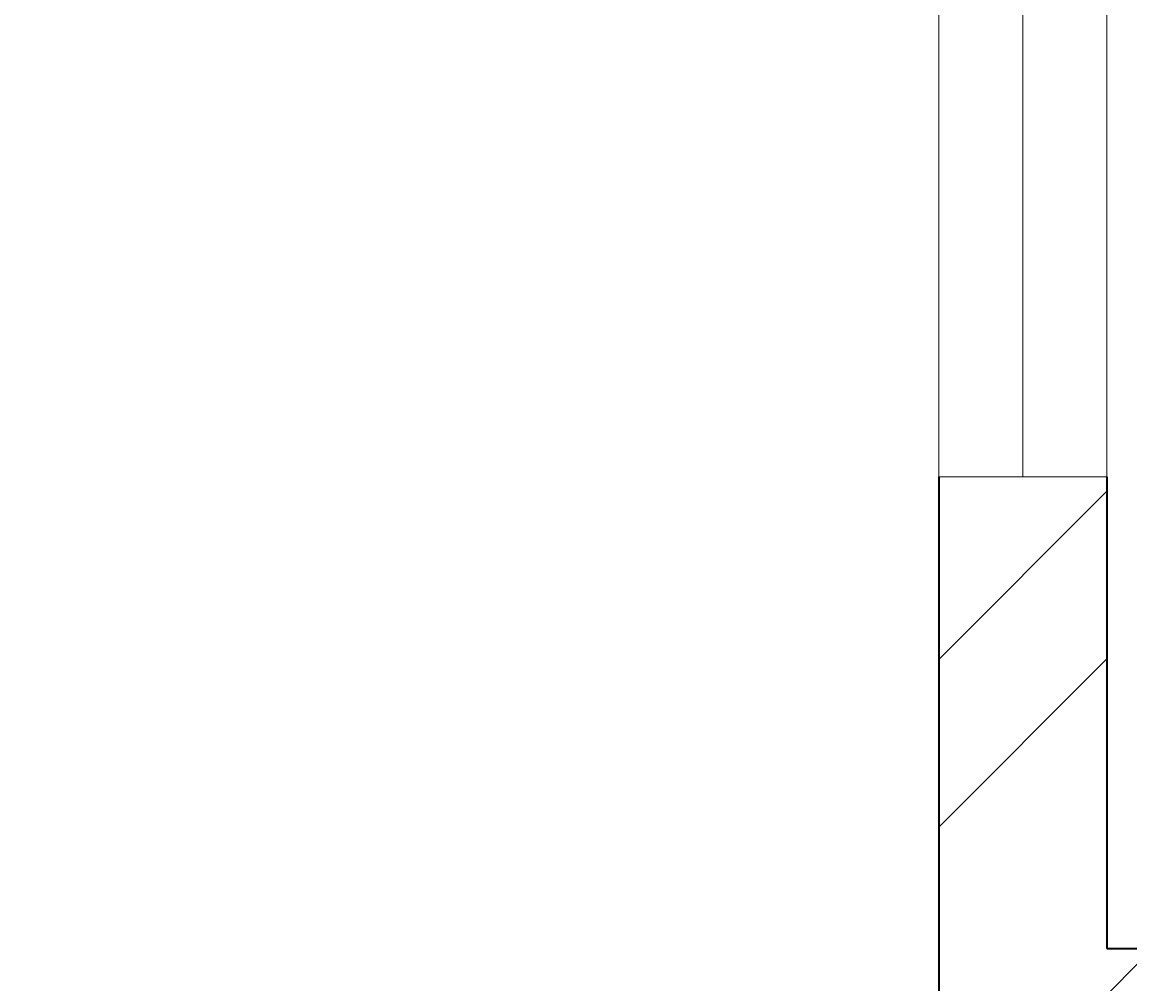
# Model space of a CAD drawing. Units: inches. Extents: x 1885 to 2748, y 783 to 2421.
# Tile 68 of 117: x 1992 to 2022, y 2022 to 2047. Entities that reach past the tile are written whole.
import ezdxf

# ---------------------------------------------------------------- set-up
doc = ezdxf.new("R2010")
doc.units = ezdxf.units.IN
for name, color, linetype, lineweight in [('A-ANNO-DIMS', 2, 'Continuous', 18), ('A-GLAZ', 181, 'Continuous', 18), ('A-WALL', 7, 'Continuous', 35)]:
    doc.layers.add(name, color=color, linetype=linetype, lineweight=lineweight)
doc.layers.add('A-WALL-PATT', color=85, linetype='Continuous', lineweight=13, true_color=0x58ba48)
doc.styles.get("Standard").update_dxf_attribs({"font": 'arial.ttf'})
doc.dimstyles.get("Standard").update_dxf_attribs({"dimtxt": 0.18, "dimasz": 0.18, "dimexe": 0.18, "dimexo": 0.0625, "dimgap": 0.09, "dimtad": 0, "dimtih": 1, "dimtoh": 1, "dimdec": 4, "dimzin": 0, "dimdsep": 46, "dimtxsty": 'Standard', "dimcen": 0.09, "dimadec": 0, "dimazin": 0, "dimtfac": 1, "dimtdec": 4, "dimtofl": 0, "dimtmove": 0, "dimatfit": 3, "dimfxl": 1, "dimtolj": 1, "dimtzin": 0, "dimarcsym": 0})

# ---------------------------------------------------------------- blocks, each defined once
blk = doc.blocks.new('*D48')
at = {"layer": 'A-ANNO-DIMS', "color": 0, "lineweight": -2, "transparency": 16777216}
for p, q in [((1980.711, 2348.006), (1902.844, 2348.006)), ((1903.024, 2347.826), (1903.024, 2114.937)), ((1903.024, 1881.686), (1903.024, 2114.574)), ((2016.711, 1881.506), (1902.844, 1881.506))]:
    blk.add_line(p, q, dxfattribs=at)
at = {"layer": 'A-ANNO-DIMS', "color": 0, "transparency": 16777216}
for points in [[(1902.994, 2347.826), (1903.054, 2347.826), (1903.024, 2348.006)], [(1902.994, 1881.686), (1903.054, 1881.686), (1903.024, 1881.506)]]:
    blk.add_solid(points, dxfattribs=at)
at = {"layer": 'Defpoints', "color": 0, "transparency": 16777216}
for p in [(1903.024, 2348.006), (1980.774, 2348.006), (2016.774, 1881.506)]:
    blk.add_point(p, dxfattribs=at)
at = {"layer": 'A-ANNO-DIMS', "color": 0, "transparency": 16777216, "insert": (1903.024, 2114.756), "char_height": 0.18, "attachment_point": 5}
blk.add_mtext('\\A1;466.5', dxfattribs=at)

msp = doc.modelspace()

# ---------------------------------------------------------------- hatches: boundary and pattern name
at = {"layer": 'A-WALL-PATT'}
h = msp.add_hatch(dxfattribs=at)
h.set_pattern_fill('ANSI32', color=256)
h.paths.add_polyline_path([(2007.772, 2318.006), (1980.774, 2318.006), (1980.774, 2281.215), (1985.274, 2281.215), (1985.274, 2313.506), (2007.772, 2313.506), (2007.772, 2315.756)])
h.paths.add_polyline_path([(2094.324, 2318.006), (2067.772, 2318.006), (2067.772, 2313.506), (2094.324, 2313.506), (2094.324, 2315.756)])
h.paths.add_polyline_path([(2131.367, 2315.756), (2131.367, 2318.006), (2131.189, 2318.006), (2112.609, 2318.006), (2112.609, 2313.506), (2117.274, 2313.506), (2117.274, 2255.201), (2121.774, 2255.201), (2121.774, 2313.506), (2131.367, 2313.506)])
h.paths.add_polyline_path([(2190.512, 2318.006), (2155.367, 2318.006), (2155.367, 2313.506), (2169.774, 2313.506), (2169.774, 2229.506), (2121.774, 2229.506), (2121.774, 2233.451), (2119.524, 2233.451), (2117.274, 2233.451), (2117.274, 2201.101), (2121.774, 2201.101), (2121.774, 2225.006), (2169.774, 2225.006), (2169.774, 2165.006), (2306.274, 2165.006), (2306.274, 2066.006), (2310.774, 2066.006), (2344.274, 2066.006), (2486.274, 2066.006), (2486.274, 1886.006), (2483.02, 1886.006), (2483.02, 1881.506), (2486.274, 1881.506), (2486.274, 1880.678), (2490.774, 1880.678), (2490.774, 2070.506), (2344.274, 2070.506), (2310.774, 2070.506), (2310.774, 2165.006), (2310.774, 2173.636), (2308.524, 2173.636), (2306.274, 2173.636), (2306.274, 2169.506), (2174.274, 2169.506), (2174.274, 2313.506), (2190.512, 2313.506), (2190.512, 2315.756)])
h.paths.add_polyline_path([(1985.274, 2221.215), (1980.774, 2221.215), (1980.774, 2165.006), (1992.774, 2165.006), (1992.774, 2141.927), (1997.274, 2141.927), (1997.274, 2165.006), (2117.274, 2165.006), (2117.274, 2163.126), (2121.774, 2163.126), (2121.774, 2172.734), (2119.524, 2172.734), (2117.274, 2172.734), (2117.274, 2169.506), (1985.274, 2169.506)])
h.paths.add_polyline_path([(1997.274, 2105.927), (1992.774, 2105.927), (1992.774, 2070.506), (2016.774, 2070.506), (2016.774, 2059.123), (2019.024, 2059.123), (2021.274, 2059.123), (2021.274, 2070.506), (2117.274, 2070.506), (2117.274, 2022.506), (2114.423, 2022.506), (2114.423, 2018.006), (2123.627, 2018.006), (2123.627, 2020.256), (2123.627, 2022.506), (2121.774, 2022.506), (2121.774, 2142.587), (2119.524, 2142.587), (2117.274, 2142.587), (2117.274, 2075.006), (1997.274, 2075.006)])
h.paths.add_polyline_path([(2092.029, 2020.256), (2092.029, 2022.506), (2021.274, 2022.506), (2021.274, 2035.123), (2016.774, 2035.123), (2016.774, 2018.006), (2016.774, 1978.784), (2021.274, 1978.784), (2021.274, 2018.006), (2092.029, 2018.006)])
h.paths.add_polyline_path([(2260.938, 2022.506), (2153.105, 2022.506), (2153.105, 2020.256), (2153.105, 2018.006), (2155.274, 2018.006), (2155.274, 1886.006), (2107.629, 1886.006), (2107.629, 1881.506), (2182.911, 1881.506), (2182.911, 1883.756), (2182.911, 1886.006), (2159.774, 1886.006), (2159.774, 2018.006), (2260.938, 2018.006), (2260.938, 2020.256)])
h.paths.add_polyline_path([(2047.629, 1883.756), (2047.629, 1886.006), (2021.274, 1886.006), (2021.274, 1918.784), (2019.024, 1918.784), (2016.774, 1918.784), (2016.774, 1881.506), (2047.629, 1881.506)])
h.paths.add_polyline_path([(2306.361, 1883.756), (2306.361, 1886.006), (2296.274, 1886.006), (2296.274, 1982.006), (2316.535, 1982.006), (2316.535, 1984.256), (2316.535, 1986.506), (2296.274, 1986.506), (2296.274, 2022.506), (2289.276, 2022.506), (2289.276, 2018.006), (2291.774, 2018.006), (2291.774, 1886.006), (2242.911, 1886.006), (2242.911, 1881.506), (2306.361, 1881.506)], flags=17)
h.paths.add_polyline_path([(1985.274, 1843.006), (2021.6, 1843.006), (2021.534, 1845.441), (2021.477, 1847.506), (1980.774, 1847.506), (1980.774, 1809.446), (1985.274, 1809.446)])
h.paths.add_polyline_path([(2131.482, 1845.256), (2131.482, 1847.506), (2081.534, 1847.506), (2081.534, 1843.006), (2117.274, 1843.006), (2117.274, 1784.147), (2119.524, 1784.147), (2121.774, 1784.147), (2121.774, 1843.006), (2131.482, 1843.006)])
h.paths.add_polyline_path([(2203.886, 1847.506), (2155.482, 1847.506), (2155.482, 1843.006), (2169.774, 1843.006), (2169.774, 1759.006), (2121.774, 1759.006), (2121.774, 1761.457), (2117.274, 1761.457), (2117.274, 1730.429), (2121.774, 1730.429), (2121.774, 1754.506), (2177.421, 1754.506), (2177.421, 1756.756), (2177.421, 1759.006), (2174.274, 1759.006), (2174.274, 1843.006), (2203.886, 1843.006)])
h.paths.add_polyline_path([(2335.554, 1845.256), (2335.554, 1847.506), (2239.886, 1847.506), (2239.886, 1843.006), (2306.274, 1843.006), (2306.274, 1759.006), (2199.486, 1759.006), (2199.486, 1754.506), (2310.774, 1754.506), (2310.774, 1843.006), (2335.554, 1843.006)])
h.paths.add_polyline_path([(2348.774, 2022.506), (2344.274, 2022.506), (2344.274, 1986.506), (2341.681, 1986.506), (2341.681, 1982.006), (2344.274, 1982.006), (2344.274, 1886.006), (2330.361, 1886.006), (2330.361, 1881.506), (2361.627, 1881.506), (2361.627, 1883.756), (2361.627, 1886.006), (2348.774, 1886.006)], flags=17)
h.paths.add_polyline_path([(2283.251, 2315.756), (2283.251, 2318.006), (2238.512, 2318.006), (2238.512, 2313.506), (2283.251, 2313.506)], flags=17)
h.paths.add_polyline_path([(2363.274, 2348.006), (2388.677, 2348.006), (2388.677, 2350.256), (2388.677, 2352.506), (2358.774, 2352.506), (2358.774, 2348.006), (2358.774, 2318.006), (2344.481, 2318.006), (2344.481, 2313.506), (2358.774, 2313.506), (2358.774, 2229.506), (2310.774, 2229.506), (2310.774, 2231.952), (2306.274, 2231.952), (2306.274, 2205.611), (2310.774, 2205.611), (2310.774, 2225.006), (2358.774, 2225.006), (2358.774, 2211.506), (2452.329, 2211.506), (2452.329, 2213.756), (2452.329, 2216.006), (2363.274, 2216.006), (2363.274, 2318.006)])
h.paths.add_polyline_path([(2310.774, 2313.506), (2320.481, 2313.506), (2320.481, 2315.756), (2320.481, 2318.006), (2302.728, 2318.006), (2302.728, 2313.506), (2306.274, 2313.506), (2306.274, 2251.076), (2310.774, 2251.076)], flags=17)
h.paths.add_polyline_path([(2490.774, 2352.506), (2486.274, 2352.506), (2448.677, 2352.506), (2448.677, 2348.006), (2486.274, 2348.006), (2486.274, 2318.006), (2486.274, 2216.006), (2481.78, 2216.006), (2481.78, 2211.506), (2486.274, 2211.506), (2486.274, 2165.006), (2493.289, 2165.006), (2493.289, 2167.256), (2493.289, 2169.506), (2490.774, 2169.506), (2490.774, 2313.506), (2494.429, 2313.506), (2494.429, 2318.006), (2490.774, 2318.006)])
h.paths.add_polyline_path([(2534.653, 2318.006), (2515.691, 2318.006), (2515.691, 2313.506), (2534.653, 2313.506), (2534.653, 2315.756)])
h.paths.add_polyline_path([(2618.274, 2318.006), (2594.653, 2318.006), (2594.653, 2313.506), (2613.774, 2313.506), (2613.774, 2281.706), (2618.274, 2281.706)])
h.paths.add_polyline_path([(2618.274, 2221.706), (2613.774, 2221.706), (2613.774, 2169.506), (2554.019, 2169.506), (2554.019, 2165.006), (2613.774, 2165.006), (2613.774, 2152.878), (2618.274, 2152.878)])
h.paths.add_polyline_path([(2618.274, 2128.878), (2616.024, 2128.878), (2613.774, 2128.878), (2613.774, 2117.006), (2529.774, 2117.006), (2529.774, 2165.006), (2532.848, 2165.006), (2532.848, 2169.506), (2522.867, 2169.506), (2522.867, 2165.006), (2525.274, 2165.006), (2525.274, 2117.006), (2525.274, 2112.506), (2525.274, 2108.576), (2529.774, 2108.576), (2529.774, 2112.506), (2613.774, 2112.506), (2613.774, 2080.19), (2618.274, 2080.19)])
h.paths.add_polyline_path([(2618.274, 2044.19), (2616.024, 2044.19), (2613.774, 2044.19), (2613.774, 2015.506), (2529.774, 2015.506), (2529.774, 2088.582), (2527.524, 2088.582), (2525.274, 2088.582), (2525.274, 2011.006), (2613.774, 2011.006), (2613.774, 1956.755), (2618.274, 1956.755)])
h.paths.add_polyline_path([(2618.274, 1881.506), (2618.274, 1896.755), (2613.774, 1896.755), (2613.774, 1881.506), (2613.774, 1847.506), (2592.715, 1847.506), (2592.715, 1843.006), (2613.774, 1843.006), (2613.774, 1765.006), (2613.774, 1760.506), (2609.621, 1760.506), (2609.621, 1756.006), (2613.774, 1756.006), (2613.774, 1660.006), (2608.544, 1660.006), (2608.544, 1655.506), (2613.774, 1655.506), (2613.774, 1508.158), (2618.274, 1508.158)])
h.paths.add_polyline_path([(2565.774, 1843.006), (2568.997, 1843.006), (2568.997, 1847.506), (2490.774, 1847.506), (2490.774, 1849.7), (2488.524, 1849.7), (2486.274, 1849.7), (2486.274, 1847.506), (2477.274, 1847.506), (2477.274, 1838.506), (2477.274, 1821.493), (2486.274, 1821.493), (2486.274, 1838.506), (2561.274, 1838.506), (2561.274, 1765.006), (2486.274, 1765.006), (2486.274, 1786.157), (2477.274, 1786.157), (2477.274, 1765.006), (2477.274, 1756.006), (2486.274, 1756.006), (2565.774, 1756.006), (2585.621, 1756.006), (2585.621, 1758.256), (2585.621, 1760.506), (2565.774, 1760.506), (2565.774, 1765.006)])
h.paths.add_polyline_path([(2486.274, 1651.006), (2561.274, 1651.006), (2561.274, 1567.006), (2486.274, 1567.006), (2486.274, 1591.321), (2477.274, 1591.321), (2477.274, 1567.006), (2477.274, 1558.006), (2477.274, 1555.439), (2481.774, 1555.439), (2481.774, 1558.006), (2568.653, 1558.006), (2568.653, 1560.256), (2568.653, 1562.506), (2565.774, 1562.506), (2565.774, 1655.506), (2584.544, 1655.506), (2584.544, 1657.756), (2584.544, 1660.006), (2565.774, 1660.006), (2486.274, 1660.006), (2477.274, 1660.006), (2477.274, 1651.006), (2477.274, 1632.989), (2486.274, 1632.989)])
h.paths.add_polyline_path([(2449.967, 1883.756), (2449.967, 1886.006), (2421.627, 1886.006), (2421.627, 1881.506), (2449.967, 1881.506)], flags=17)
h.paths.add_polyline_path([(2447.274, 1847.506), (2395.554, 1847.506), (2395.554, 1843.006), (2442.774, 1843.006), (2442.774, 1809.27), (2447.274, 1809.27)])
h.paths.add_polyline_path([(1985.274, 1749.446), (1980.774, 1749.446), (1980.774, 1694.504), (1985.274, 1694.504), (1985.274, 1694.506), (1986.897, 1694.506), (1986.897, 1697.78), (1986.897, 1699.006), (1985.274, 1699.006)])
h.paths.add_polyline_path([(2152.774, 1699.006), (2121.774, 1699.006), (2121.774, 1703.668), (2119.524, 1703.668), (2117.274, 1703.668), (2117.274, 1699.006), (2009.219, 1699.006), (2009.219, 1694.506), (2148.274, 1694.506), (2148.274, 1692.631), (2152.774, 1692.631)])
h.paths.add_polyline_path([(2016.274, 1694.506), (2011.774, 1694.506), (2011.774, 1558.006), (2040.806, 1558.006), (2040.806, 1560.256), (2040.806, 1562.506), (2016.274, 1562.506)])
h.paths.add_polyline_path([(2152.774, 1663.017), (2150.524, 1663.017), (2148.274, 1663.017), (2148.274, 1562.506), (2100.806, 1562.506), (2100.806, 1558.006), (2165.119, 1558.006), (2165.119, 1560.256), (2165.119, 1562.506), (2152.774, 1562.506), (2152.774, 1610.506), (2224.774, 1610.506), (2224.774, 1607.99), (2229.274, 1607.99), (2229.274, 1615.006), (2152.774, 1615.006)])
h.paths.add_polyline_path([(2238.613, 1560.256), (2238.613, 1562.506), (2229.274, 1562.506), (2229.274, 1588.756), (2227.024, 1588.763), (2224.774, 1588.771), (2224.774, 1562.506), (2189.119, 1562.506), (2189.119, 1558.006), (2238.613, 1558.006)])
h.paths.add_polyline_path([(2336.024, 1560.256), (2336.024, 1562.506), (2310.774, 1562.506), (2310.774, 1656.347), (2308.524, 1656.347), (2306.274, 1656.347), (2306.274, 1562.506), (2286.613, 1562.506), (2286.613, 1558.006), (2336.024, 1558.006)])
h.paths.add_polyline_path([(2447.274, 1690.968), (2445.024, 1690.968), (2442.774, 1690.968), (2442.774, 1687.006), (2306.274, 1687.006), (2306.274, 1680.75), (2310.774, 1680.75), (2310.774, 1682.506), (2442.774, 1682.506), (2442.774, 1562.506), (2396.024, 1562.506), (2396.024, 1558.006), (2447.274, 1558.006)])
h.paths.add_polyline_path([(2447.274, 1749.27), (2445.024, 1749.27), (2442.774, 1749.27), (2442.774, 1717.232), (2447.274, 1717.232)])
h.paths.add_polyline_path([(2044.674, 1521.756), (2044.674, 1524.006), (2007.274, 1524.006), (2007.274, 1503.49), (2009.524, 1503.49), (2011.774, 1503.49), (2011.774, 1519.506), (2044.674, 1519.506)])
h.paths.add_polyline_path([(2177.969, 1521.756), (2177.969, 1524.006), (2104.674, 1524.006), (2104.674, 1519.506), (2145.774, 1519.506), (2145.774, 1387.506), (2143.37, 1387.506), (2143.37, 1383.006), (2251.585, 1383.006), (2251.585, 1385.256), (2251.585, 1387.506), (2150.274, 1387.506), (2150.274, 1519.506), (2177.969, 1519.506)])
h.paths.add_polyline_path([(2298.704, 1524.006), (2237.969, 1524.006), (2237.969, 1519.506), (2282.274, 1519.506), (2282.274, 1387.506), (2279.683, 1387.506), (2279.683, 1383.006), (2286.774, 1383.006), (2286.774, 1419.006), (2312.451, 1419.006), (2312.451, 1421.256), (2312.451, 1423.506), (2286.774, 1423.506), (2286.774, 1519.506), (2298.704, 1519.506), (2298.704, 1521.722)], flags=17)
h.paths.add_polyline_path([(2361.897, 1521.756), (2361.897, 1524.006), (2322.704, 1524.006), (2322.704, 1519.506), (2334.774, 1519.506), (2334.774, 1423.506), (2331.93, 1423.506), (2331.93, 1419.006), (2334.774, 1419.006), (2334.774, 1387.506), (2334.774, 1383.228), (2339.274, 1383.228), (2339.274, 1387.506), (2339.274, 1519.506), (2361.897, 1519.506)], flags=17)
h.paths.add_polyline_path([(2447.274, 1521.756), (2447.274, 1524.006), (2421.897, 1524.006), (2421.897, 1519.506), (2447.274, 1519.506)], flags=17)
h.paths.add_polyline_path([(2481.774, 1529.6), (2479.524, 1529.6), (2477.274, 1529.6), (2477.274, 1524.006), (2474.489, 1524.006), (2474.489, 1519.506), (2477.274, 1519.506), (2477.274, 1334.506), (2296.774, 1334.506), (2296.774, 1240.506), (2160.274, 1240.506), (2160.274, 1180.506), (2112.274, 1180.506), (2112.274, 1207.692), (2110.024, 1207.692), (2107.774, 1207.692), (2107.774, 1171.609), (2112.274, 1171.609), (2112.274, 1176.006), (2160.274, 1176.006), (2160.274, 1092.006), (2144.221, 1092.006), (2144.221, 1087.506), (2189.497, 1087.506), (2189.497, 1089.756), (2189.497, 1092.006), (2164.774, 1092.006), (2164.774, 1236.006), (2296.774, 1236.006), (2296.774, 1231.912), (2301.274, 1231.912), (2301.274, 1330.006), (2481.774, 1330.006), (2481.774, 1387.506)])
h.paths.add_polyline_path([(2618.274, 1448.158), (2613.774, 1448.158), (2613.774, 1382.506), (2529.774, 1382.506), (2525.274, 1382.506), (2525.274, 1307.062), (2529.774, 1307.062), (2529.774, 1378.006), (2613.774, 1378.006), (2613.774, 1354.988), (2618.274, 1354.988)])
h.paths.add_polyline_path([(2618.274, 1318.988), (2613.774, 1318.988), (2613.774, 1281.006), (2529.774, 1281.006), (2529.774, 1283.786), (2527.524, 1283.786), (2525.274, 1283.786), (2525.274, 1228.506), (2516.794, 1228.506), (2516.794, 1224.006), (2533.484, 1224.006), (2533.484, 1226.256), (2533.484, 1228.506), (2529.774, 1228.506), (2529.774, 1276.506), (2613.774, 1276.506), (2613.774, 1266.02), (2618.274, 1266.02)])
h.paths.add_polyline_path([(2618.274, 1134.964), (2613.774, 1134.964), (2613.774, 1092.006), (2594.545, 1092.006), (2594.545, 1087.506), (2618.274, 1087.506)])
h.paths.add_polyline_path([(2534.545, 1092.006), (2509.765, 1092.006), (2509.765, 1087.506), (2534.545, 1087.506), (2534.545, 1089.756)])
h.paths.add_polyline_path([(2481.274, 1224.006), (2484.117, 1224.006), (2484.117, 1226.256), (2484.117, 1228.506), (2476.774, 1228.506), (2476.774, 1198.506), (2471.61, 1198.506), (2471.61, 1194.006), (2476.774, 1194.006), (2476.774, 1062.006), (2436.894, 1062.006), (2436.894, 1057.506), (2476.774, 1057.506), (2481.274, 1057.506), (2481.274, 1062.006), (2481.274, 1087.506), (2485.354, 1087.506), (2485.354, 1089.756), (2485.354, 1092.006), (2481.274, 1092.006), (2481.274, 1117.506)])
h.paths.add_polyline_path([(2439.898, 1198.506), (2349.274, 1198.506), (2349.274, 1194.006), (2349.274, 1180.506), (2301.274, 1180.506), (2301.274, 1201.896), (2299.024, 1201.896), (2296.774, 1201.896), (2296.774, 1172.335), (2299.024, 1172.335), (2301.274, 1172.335), (2301.274, 1176.006), (2349.274, 1176.006), (2349.274, 1092.006), (2334.452, 1092.006), (2334.452, 1087.506), (2349.274, 1087.506), (2349.274, 1057.506), (2353.774, 1057.506), (2376.894, 1057.506), (2376.894, 1059.756), (2376.894, 1062.006), (2353.774, 1062.006), (2353.774, 1087.506), (2353.774, 1180.506), (2353.774, 1194.006), (2439.898, 1194.006), (2439.898, 1196.256)])
h.paths.add_polyline_path([(2270.596, 1089.756), (2270.596, 1092.006), (2249.497, 1092.006), (2249.497, 1087.506), (2270.596, 1087.506)], flags=17)
h.paths.add_polyline_path([(2310.452, 1092.006), (2301.274, 1092.006), (2301.274, 1153.292), (2296.774, 1153.292), (2296.774, 1092.006), (2293.786, 1092.006), (2293.786, 1087.506), (2310.452, 1087.506), (2310.452, 1089.756)], flags=17)
h.paths.add_polyline_path([(2112.274, 1150.328), (2110.024, 1150.328), (2107.774, 1150.328), (2107.774, 1092.006), (2104.465, 1092.006), (2104.465, 1087.506), (2120.221, 1087.506), (2120.221, 1089.756), (2120.221, 1092.006), (2112.274, 1092.006)])
h.paths.add_polyline_path([(2082.172, 1092.006), (2058.144, 1092.006), (2058.144, 1087.506), (2082.172, 1087.506), (2082.172, 1089.756)])
h.paths.add_polyline_path([(1975.774, 1145.638), (1971.274, 1145.638), (1971.274, 1087.506), (1980.774, 1087.506), (1998.144, 1087.506), (1998.144, 1089.756), (1998.144, 1092.006), (1985.274, 1092.006), (1975.774, 1092.006)])
h.paths.add_polyline_path([(2112.274, 1244.385), (2110.024, 1244.385), (2107.774, 1244.385), (2107.774, 1240.506), (1992.274, 1240.506), (1992.274, 1271.008), (1987.774, 1271.008), (1987.774, 1240.506), (1980.774, 1240.506), (1975.774, 1240.506), (1971.274, 1240.506), (1971.274, 1205.638), (1975.774, 1205.638), (1975.774, 1236.006), (2107.774, 1236.006), (2107.774, 1233.444), (2112.274, 1233.444), (2112.274, 1236.006)])
h.paths.add_polyline_path([(2112.274, 1383.006), (2114.783, 1383.006), (2114.783, 1385.256), (2114.783, 1387.506), (2102.476, 1387.506), (2102.476, 1383.006), (2107.774, 1383.006), (2107.774, 1335.006), (2011.774, 1335.006), (2011.774, 1349.939), (2007.274, 1349.939), (2007.274, 1335.006), (1987.774, 1335.006), (1987.774, 1330.506), (1987.774, 1307.008), (1992.274, 1307.008), (1992.274, 1330.506), (2007.274, 1330.506), (2107.774, 1330.506), (2107.774, 1264.711), (2112.274, 1264.711)])
h.paths.add_polyline_path([(2077.857, 1387.506), (2011.774, 1387.506), (2011.774, 1390.036), (2009.524, 1390.036), (2007.274, 1390.036), (2007.274, 1373.939), (2011.774, 1373.939), (2011.774, 1383.006), (2077.857, 1383.006)])
h.paths.add_polyline_path([(2011.774, 1443.49), (2007.274, 1443.49), (2007.274, 1410.248), (2011.774, 1410.248)])

# ---------------------------------------------------------------- linework, layer by layer
at = {"layer": 'A-GLAZ'}
for p, q in [((2016.774, 2059.123), (2016.774, 2035.123)), ((2019.024, 2059.123), (2019.024, 2035.123)), ((2021.274, 2035.123), (2021.274, 2059.123)), ((2019.024, 2035.123), (2016.774, 2035.123)), ((2016.774, 2035.123), (2021.274, 2035.123))]:
    msp.add_line(p, q, dxfattribs=at)
at = {"layer": 'A-WALL'}
for p, q in [((2016.774, 2035.123), (2016.774, 2018.006)), ((2021.274, 2035.123), (2021.274, 2022.506)), ((2021.274, 2022.506), (2093.567, 2022.506))]:
    msp.add_line(p, q, dxfattribs=at)

# ---------------------------------------------------------------- dimensions: what is measured, and where the dimension line sits
at = {"layer": 'A-ANNO-DIMS'}
dim = msp.add_linear_dim(base=(1903.024, 2348.006), p1=(2016.774, 1881.506), p2=(1980.774, 2348.006), angle=90, dimstyle='Standard', override={"dimdec": 1, "dimlfac": 1, "dimrnd": 0, "dimzin": 0, "dimdsep": 46, "dimlunit": 2}, dxfattribs=at)
dim.commit()
dim.dimension.update_dxf_attribs({"geometry": '*D48', "text_midpoint": (1903.024, 2114.756)})

doc.saveas('drawing.dxf')
